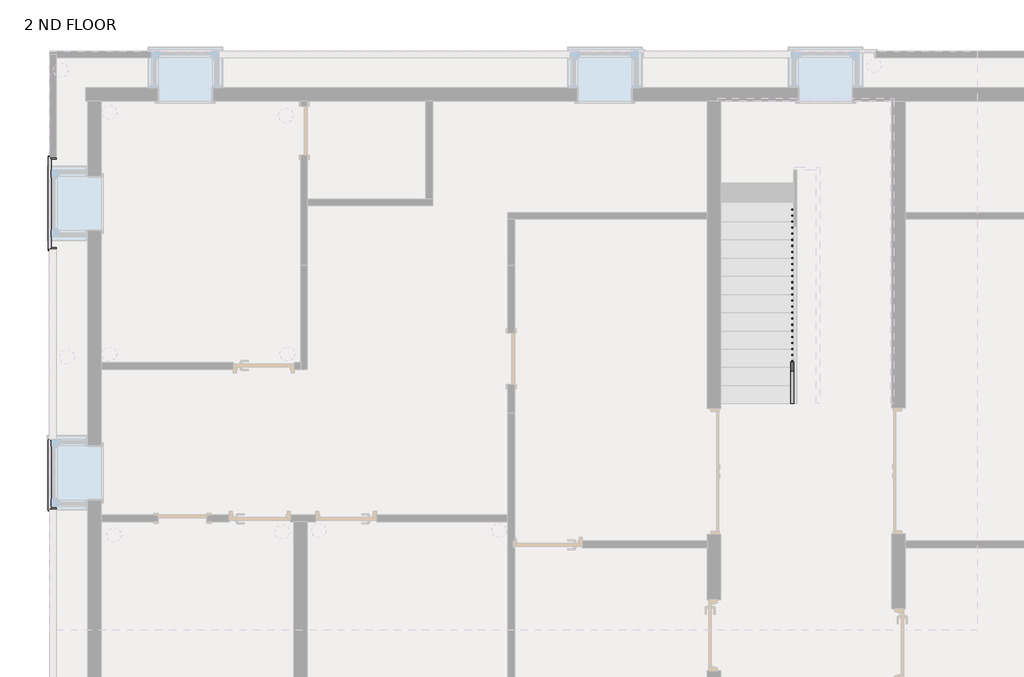
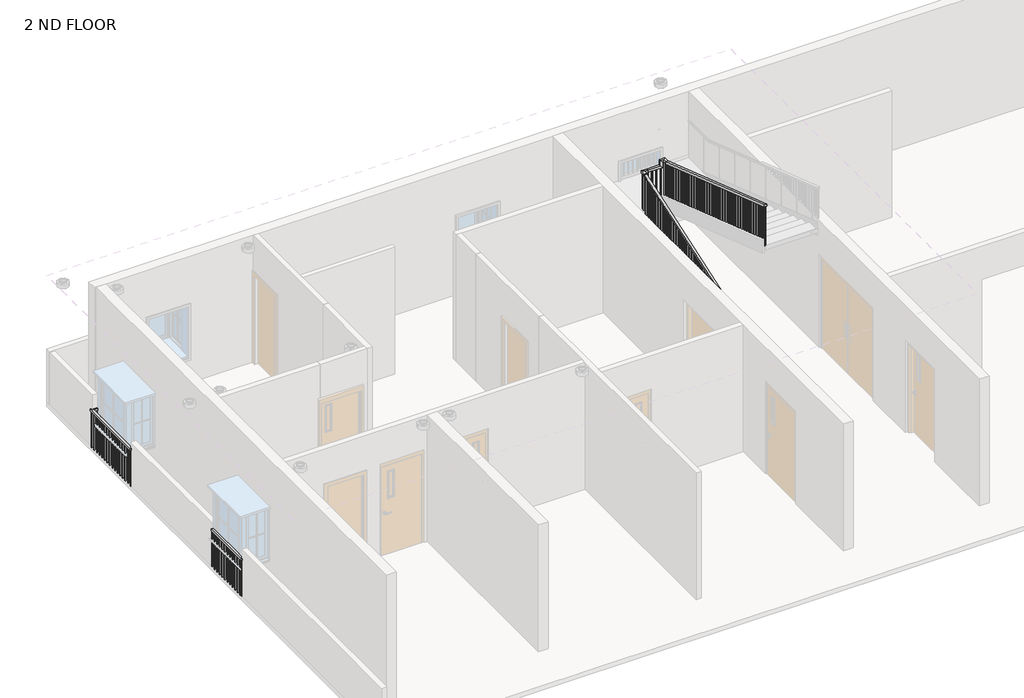
# One storey, part 4 of 7: 3 railings.
"""IFC4 building model written with IfcOpenShell, lengths in millimetres."""

from ifc_helpers import new_model, si_unit, frame, origin, place, context, project, spatial, polyline, outline, extrude, faceted_brep, element, save

model = new_model("IFC4")

# Units and contexts
model_context = context("Model", 3, world=origin())
ifc_project = project(units=[si_unit("LENGTHUNIT", "METRE", prefix="MILLI")], contexts=[model_context])

# Site, building, storey
site = spatial("IfcSite", under=ifc_project)
building = spatial("IfcBuilding", under=site)
storey = spatial("IfcBuildingStorey", under=building, Name="2 ND FLOOR", Elevation=6400.8)

# Railings
placement = place(None, origin())
element("IfcRailing", 1, ObjectType="Handrail - Rectangular", at=placement, inside=storey, context=model_context, shape_type="SolidModel", body=[
    faceted_brep([(-680.3987998, 2564.5067329, 7418.6142857), (-680.3987998, 2564.5067329, 7364.9699957), (-629.5987998, 2564.5067329, 7364.9699957), (-629.5987998, 2564.5067329, 7418.6142857), (-680.3987998, 6450.7067329, 8737.1464286), (-680.3987998, 6501.5067329, 8700.7378529), (-629.5987998, 6501.5067329, 8700.7378529), (-629.5987998, 6450.7067329, 8737.1464286), (-553.3987998, 6577.7067329, 8712.2), (-553.3987998, 6577.7067329, 8763.0), (-273.9987915, 6577.7067329, 8763.0), (-223.1987915, 6577.7067329, 8712.2), (-553.3987998, 6526.9067329, 8712.2), (-223.1987915, 6526.9067329, 8712.2), (-553.3987998, 6526.9067329, 8763.0), (-273.9987915, 6526.9067329, 8763.0), (-146.9987915, 2564.5067329, 10210.8), (-197.7987915, 2564.5067329, 10210.8), (-197.7987915, 2564.5067329, 10157.15571), (-146.9987915, 2564.5067329, 10157.15571), (-146.9987915, 6442.3235624, 8841.4678571), (-146.9987915, 6450.7067329, 8892.2678571), (-197.7987915, 6442.3235624, 8841.4678571), (-197.7987915, 6450.7067329, 8892.2678571), (-680.3987998, 6450.7067329, 8763.0), (-680.3987998, 6501.5067329, 8712.2), (-629.5987998, 6501.5067329, 8712.2), (-629.5987998, 6450.7067329, 8763.0), (-680.3987998, 6577.7067329, 8763.0), (-680.3987998, 6577.7067329, 8712.2), (-629.5987998, 6526.9067329, 8712.2), (-629.5987998, 6526.9067329, 8763.0), (-273.9987915, 6577.7067329, 8892.2678571), (-223.1987915, 6577.7067329, 8841.4678571), (-223.1987915, 6526.9067329, 8841.4678571), (-273.9987915, 6526.9067329, 8892.2678571), (-146.9987915, 6577.7067329, 8892.2678571), (-146.9987915, 6577.7067329, 8841.4678571), (-197.7987915, 6526.9067329, 8841.4678571), (-197.7987915, 6526.9067329, 8892.2678571)], [[[0, 1, 2, 3]], [[1, 0, 4, 5]], [[2, 1, 5, 6]], [[3, 2, 6, 7]], [[0, 3, 7, 4]], [[8, 9, 10, 11]], [[12, 8, 11, 13]], [[14, 12, 13, 15]], [[9, 14, 15, 10]], [[16, 17, 18, 19]], [[20, 21, 16, 19]], [[22, 20, 19, 18]], [[23, 22, 18, 17]], [[21, 23, 17, 16]], [[5, 4, 24, 25]], [[6, 5, 25, 26]], [[7, 6, 26, 27]], [[4, 7, 27, 24]], [[25, 24, 28, 29]], [[26, 25, 29, 30]], [[27, 26, 30, 31]], [[24, 27, 31, 28]], [[29, 28, 9, 8]], [[30, 29, 8, 12]], [[31, 30, 12, 14]], [[28, 31, 14, 9]], [[11, 10, 32, 33]], [[13, 11, 33, 34]], [[15, 13, 34, 35]], [[10, 15, 35, 32]], [[33, 32, 36, 37]], [[34, 33, 37, 38]], [[35, 34, 38, 39]], [[32, 35, 39, 36]], [[37, 36, 21, 20]], [[38, 37, 20, 22]], [[39, 38, 22, 23]], [[36, 39, 23, 21]]]),
    extrude(outline(polyline([(2580.3817329, 10151.7695493), (2599.4317329, 10145.3061565), (2599.4317329, 9192.9857143), (2580.3817329, 9192.9857143), (2580.3817329, 10151.7695493)])), frame((-181.9237915, 0.0, 0.0), z_axis=(1.0, 0.0, 0.0), x_axis=(0.0, 1.0, 0.0)), (0.0, 0.0, 1.0), 19.05),
    extrude(outline(polyline([(2681.9817329, 10117.2981207), (2701.0317329, 10110.8347279), (2701.0317329, 9192.9857143), (2681.9817329, 9192.9857143), (2681.9817329, 10117.2981207)])), frame((-181.9237915, 0.0, 0.0), z_axis=(1.0, 0.0, 0.0), x_axis=(0.0, 1.0, 0.0)), (0.0, 0.0, 1.0), 19.05),
    extrude(outline(polyline([(2783.5817329, 10082.8266922), (2802.6317329, 10076.3632993), (2802.6317329, 9192.9857143), (2783.5817329, 9192.9857143), (2783.5817329, 10082.8266922)])), frame((-181.9237915, 0.0, 0.0), z_axis=(1.0, 0.0, 0.0), x_axis=(0.0, 1.0, 0.0)), (0.0, 0.0, 1.0), 19.05),
    extrude(outline(polyline([(2885.1817329, 10048.3552636), (2904.2317329, 10041.8918707), (2904.2317329, 9089.5714286), (2885.1817329, 9089.5714286), (2885.1817329, 10048.3552636)])), frame((-181.9237915, 0.0, 0.0), z_axis=(1.0, 0.0, 0.0), x_axis=(0.0, 1.0, 0.0)), (0.0, 0.0, 1.0), 19.05),
    extrude(outline(polyline([(2986.7817329, 10013.883835), (3005.8317329, 10007.4204422), (3005.8317329, 9089.5714286), (2986.7817329, 9089.5714286), (2986.7817329, 10013.883835)])), frame((-181.9237915, 0.0, 0.0), z_axis=(1.0, 0.0, 0.0), x_axis=(0.0, 1.0, 0.0)), (0.0, 0.0, 1.0), 19.05),
    extrude(outline(polyline([(3088.3817329, 9979.4124065), (3107.4317329, 9972.9490136), (3107.4317329, 9089.5714286), (3088.3817329, 9089.5714286), (3088.3817329, 9979.4124065)])), frame((-181.9237915, 0.0, 0.0), z_axis=(1.0, 0.0, 0.0), x_axis=(0.0, 1.0, 0.0)), (0.0, 0.0, 1.0), 19.05),
    extrude(outline(polyline([(3189.9817329, 9944.9409779), (3209.0317329, 9938.477585), (3209.0317329, 8986.1571429), (3189.9817329, 8986.1571429), (3189.9817329, 9944.9409779)])), frame((-181.9237915, 0.0, 0.0), z_axis=(1.0, 0.0, 0.0), x_axis=(0.0, 1.0, 0.0)), (0.0, 0.0, 1.0), 19.05),
    extrude(outline(polyline([(3291.5817329, 9910.4695493), (3310.6317329, 9904.0061565), (3310.6317329, 8986.1571429), (3291.5817329, 8986.1571429), (3291.5817329, 9910.4695493)])), frame((-181.9237915, 0.0, 0.0), z_axis=(1.0, 0.0, 0.0), x_axis=(0.0, 1.0, 0.0)), (0.0, 0.0, 1.0), 19.05),
    extrude(outline(polyline([(3393.1817329, 9875.9981207), (3412.2317329, 9869.5347279), (3412.2317329, 8986.1571429), (3393.1817329, 8986.1571429), (3393.1817329, 9875.9981207)])), frame((-181.9237915, 0.0, 0.0), z_axis=(1.0, 0.0, 0.0), x_axis=(0.0, 1.0, 0.0)), (0.0, 0.0, 1.0), 19.05),
    extrude(outline(polyline([(3494.7817329, 9841.5266922), (3513.8317329, 9835.0632993), (3513.8317329, 8882.7428571), (3494.7817329, 8882.7428571), (3494.7817329, 9841.5266922)])), frame((-181.9237915, 0.0, 0.0), z_axis=(1.0, 0.0, 0.0), x_axis=(0.0, 1.0, 0.0)), (0.0, 0.0, 1.0), 19.05),
    extrude(outline(polyline([(3596.3817329, 9807.0552636), (3615.4317329, 9800.5918707), (3615.4317329, 8882.7428571), (3596.3817329, 8882.7428571), (3596.3817329, 9807.0552636)])), frame((-181.9237915, 0.0, 0.0), z_axis=(1.0, 0.0, 0.0), x_axis=(0.0, 1.0, 0.0)), (0.0, 0.0, 1.0), 19.05),
    extrude(outline(polyline([(3697.9817329, 9772.583835), (3717.0317329, 9766.1204422), (3717.0317329, 8882.7428571), (3697.9817329, 8882.7428571), (3697.9817329, 9772.583835)])), frame((-181.9237915, 0.0, 0.0), z_axis=(1.0, 0.0, 0.0), x_axis=(0.0, 1.0, 0.0)), (0.0, 0.0, 1.0), 19.05),
    extrude(outline(polyline([(3799.5817329, 9738.1124065), (3818.6317329, 9731.6490136), (3818.6317329, 8779.3285714), (3799.5817329, 8779.3285714), (3799.5817329, 9738.1124065)])), frame((-181.9237915, 0.0, 0.0), z_axis=(1.0, 0.0, 0.0), x_axis=(0.0, 1.0, 0.0)), (0.0, 0.0, 1.0), 19.05),
    extrude(outline(polyline([(3901.1817329, 9703.6409779), (3920.2317329, 9697.177585), (3920.2317329, 8779.3285714), (3901.1817329, 8779.3285714), (3901.1817329, 9703.6409779)])), frame((-181.9237915, 0.0, 0.0), z_axis=(1.0, 0.0, 0.0), x_axis=(0.0, 1.0, 0.0)), (0.0, 0.0, 1.0), 19.05),
    extrude(outline(polyline([(4002.7817329, 9669.1695493), (4021.8317329, 9662.7061565), (4021.8317329, 8779.3285714), (4002.7817329, 8779.3285714), (4002.7817329, 9669.1695493)])), frame((-181.9237915, 0.0, 0.0), z_axis=(1.0, 0.0, 0.0), x_axis=(0.0, 1.0, 0.0)), (0.0, 0.0, 1.0), 19.05),
    extrude(outline(polyline([(4104.3817329, 9634.6981207), (4123.4317329, 9628.2347279), (4123.4317329, 8675.9142857), (4104.3817329, 8675.9142857), (4104.3817329, 9634.6981207)])), frame((-181.9237915, 0.0, 0.0), z_axis=(1.0, 0.0, 0.0), x_axis=(0.0, 1.0, 0.0)), (0.0, 0.0, 1.0), 19.05),
    extrude(outline(polyline([(4205.9817329, 9600.2266922), (4225.0317329, 9593.7632993), (4225.0317329, 8675.9142857), (4205.9817329, 8675.9142857), (4205.9817329, 9600.2266922)])), frame((-181.9237915, 0.0, 0.0), z_axis=(1.0, 0.0, 0.0), x_axis=(0.0, 1.0, 0.0)), (0.0, 0.0, 1.0), 19.05),
    extrude(outline(polyline([(4307.5817329, 9565.7552636), (4326.6317329, 9559.2918707), (4326.6317329, 8675.9142857), (4307.5817329, 8675.9142857), (4307.5817329, 9565.7552636)])), frame((-181.9237915, 0.0, 0.0), z_axis=(1.0, 0.0, 0.0), x_axis=(0.0, 1.0, 0.0)), (0.0, 0.0, 1.0), 19.05),
    extrude(outline(polyline([(4409.1817329, 9531.283835), (4428.2317329, 9524.8204422), (4428.2317329, 8572.5), (4409.1817329, 8572.5), (4409.1817329, 9531.283835)])), frame((-181.9237915, 0.0, 0.0), z_axis=(1.0, 0.0, 0.0), x_axis=(0.0, 1.0, 0.0)), (0.0, 0.0, 1.0), 19.05),
    extrude(outline(polyline([(4510.7817329, 9496.8124065), (4529.8317329, 9490.3490136), (4529.8317329, 8572.5), (4510.7817329, 8572.5), (4510.7817329, 9496.8124065)])), frame((-181.9237915, 0.0, 0.0), z_axis=(1.0, 0.0, 0.0), x_axis=(0.0, 1.0, 0.0)), (0.0, 0.0, 1.0), 19.05),
    extrude(outline(polyline([(4612.3817329, 9462.3409779), (4631.4317329, 9455.877585), (4631.4317329, 8572.5), (4612.3817329, 8572.5), (4612.3817329, 9462.3409779)])), frame((-181.9237915, 0.0, 0.0), z_axis=(1.0, 0.0, 0.0), x_axis=(0.0, 1.0, 0.0)), (0.0, 0.0, 1.0), 19.05),
    extrude(outline(polyline([(4713.9817329, 9427.8695493), (4733.0317329, 9421.4061565), (4733.0317329, 8469.0857143), (4713.9817329, 8469.0857143), (4713.9817329, 9427.8695493)])), frame((-181.9237915, 0.0, 0.0), z_axis=(1.0, 0.0, 0.0), x_axis=(0.0, 1.0, 0.0)), (0.0, 0.0, 1.0), 19.05),
    extrude(outline(polyline([(4815.5817329, 9393.3981207), (4834.6317329, 9386.9347279), (4834.6317329, 8469.0857143), (4815.5817329, 8469.0857143), (4815.5817329, 9393.3981207)])), frame((-181.9237915, 0.0, 0.0), z_axis=(1.0, 0.0, 0.0), x_axis=(0.0, 1.0, 0.0)), (0.0, 0.0, 1.0), 19.05),
    extrude(outline(polyline([(4917.1817329, 9358.9266922), (4936.2317329, 9352.4632993), (4936.2317329, 8469.0857143), (4917.1817329, 8469.0857143), (4917.1817329, 9358.9266922)])), frame((-181.9237915, 0.0, 0.0), z_axis=(1.0, 0.0, 0.0), x_axis=(0.0, 1.0, 0.0)), (0.0, 0.0, 1.0), 19.05),
    extrude(outline(polyline([(5018.7817329, 9324.4552636), (5037.8317329, 9317.9918707), (5037.8317329, 8365.6714286), (5018.7817329, 8365.6714286), (5018.7817329, 9324.4552636)])), frame((-181.9237915, 0.0, 0.0), z_axis=(1.0, 0.0, 0.0), x_axis=(0.0, 1.0, 0.0)), (0.0, 0.0, 1.0), 19.05),
    extrude(outline(polyline([(5120.3817329, 9289.983835), (5139.4317329, 9283.5204422), (5139.4317329, 8365.6714286), (5120.3817329, 8365.6714286), (5120.3817329, 9289.983835)])), frame((-181.9237915, 0.0, 0.0), z_axis=(1.0, 0.0, 0.0), x_axis=(0.0, 1.0, 0.0)), (0.0, 0.0, 1.0), 19.05),
    extrude(outline(polyline([(5221.9817329, 9255.5124065), (5241.0317329, 9249.0490136), (5241.0317329, 8365.6714286), (5221.9817329, 8365.6714286), (5221.9817329, 9255.5124065)])), frame((-181.9237915, 0.0, 0.0), z_axis=(1.0, 0.0, 0.0), x_axis=(0.0, 1.0, 0.0)), (0.0, 0.0, 1.0), 19.05),
    extrude(outline(polyline([(5323.5817329, 9221.0409779), (5342.6317329, 9214.577585), (5342.6317329, 8262.2571429), (5323.5817329, 8262.2571429), (5323.5817329, 9221.0409779)])), frame((-181.9237915, 0.0, 0.0), z_axis=(1.0, 0.0, 0.0), x_axis=(0.0, 1.0, 0.0)), (0.0, 0.0, 1.0), 19.05),
    extrude(outline(polyline([(5425.1817329, 9186.5695493), (5444.2317329, 9180.1061565), (5444.2317329, 8262.2571429), (5425.1817329, 8262.2571429), (5425.1817329, 9186.5695493)])), frame((-181.9237915, 0.0, 0.0), z_axis=(1.0, 0.0, 0.0), x_axis=(0.0, 1.0, 0.0)), (0.0, 0.0, 1.0), 19.05),
    extrude(outline(polyline([(5526.7817329, 9152.0981207), (5545.8317329, 9145.6347279), (5545.8317329, 8262.2571429), (5526.7817329, 8262.2571429), (5526.7817329, 9152.0981207)])), frame((-181.9237915, 0.0, 0.0), z_axis=(1.0, 0.0, 0.0), x_axis=(0.0, 1.0, 0.0)), (0.0, 0.0, 1.0), 19.05),
    extrude(outline(polyline([(5628.3817329, 9117.6266922), (5647.4317329, 9111.1632993), (5647.4317329, 8158.8428571), (5628.3817329, 8158.8428571), (5628.3817329, 9117.6266922)])), frame((-181.9237915, 0.0, 0.0), z_axis=(1.0, 0.0, 0.0), x_axis=(0.0, 1.0, 0.0)), (0.0, 0.0, 1.0), 19.05),
    extrude(outline(polyline([(5729.9817329, 9083.1552636), (5749.0317329, 9076.6918707), (5749.0317329, 8158.8428571), (5729.9817329, 8158.8428571), (5729.9817329, 9083.1552636)])), frame((-181.9237915, 0.0, 0.0), z_axis=(1.0, 0.0, 0.0), x_axis=(0.0, 1.0, 0.0)), (0.0, 0.0, 1.0), 19.05),
    extrude(outline(polyline([(5831.5817329, 9048.683835), (5850.6317329, 9042.2204422), (5850.6317329, 8158.8428571), (5831.5817329, 8158.8428571), (5831.5817329, 9048.683835)])), frame((-181.9237915, 0.0, 0.0), z_axis=(1.0, 0.0, 0.0), x_axis=(0.0, 1.0, 0.0)), (0.0, 0.0, 1.0), 19.05),
    extrude(outline(polyline([(5933.1817329, 9014.2124065), (5952.2317329, 9007.7490136), (5952.2317329, 8055.4285714), (5933.1817329, 8055.4285714), (5933.1817329, 9014.2124065)])), frame((-181.9237915, 0.0, 0.0), z_axis=(1.0, 0.0, 0.0), x_axis=(0.0, 1.0, 0.0)), (0.0, 0.0, 1.0), 19.05),
    extrude(outline(polyline([(6034.7817329, 8979.7409779), (6053.8317329, 8973.277585), (6053.8317329, 8055.4285714), (6034.7817329, 8055.4285714), (6034.7817329, 8979.7409779)])), frame((-181.9237915, 0.0, 0.0), z_axis=(1.0, 0.0, 0.0), x_axis=(0.0, 1.0, 0.0)), (0.0, 0.0, 1.0), 19.05),
    extrude(outline(polyline([(6136.3817329, 8945.2695493), (6155.4317329, 8938.8061565), (6155.4317329, 8055.4285714), (6136.3817329, 8055.4285714), (6136.3817329, 8945.2695493)])), frame((-181.9237915, 0.0, 0.0), z_axis=(1.0, 0.0, 0.0), x_axis=(0.0, 1.0, 0.0)), (0.0, 0.0, 1.0), 19.05),
    extrude(outline(polyline([(6237.9817329, 8910.7981207), (6257.0317329, 8904.3347279), (6257.0317329, 7952.0142857), (6237.9817329, 7952.0142857), (6237.9817329, 8910.7981207)])), frame((-181.9237915, 0.0, 0.0), z_axis=(1.0, 0.0, 0.0), x_axis=(0.0, 1.0, 0.0)), (0.0, 0.0, 1.0), 19.05),
    extrude(outline(polyline([(6339.5817329, 8876.3266922), (6358.6317329, 8869.8632993), (6358.6317329, 7952.0142857), (6339.5817329, 7952.0142857), (6339.5817329, 8876.3266922)])), frame((-181.9237915, 0.0, 0.0), z_axis=(1.0, 0.0, 0.0), x_axis=(0.0, 1.0, 0.0)), (0.0, 0.0, 1.0), 19.05),
    extrude(outline(polyline([(6441.1817329, 8841.8552636), (6460.2317329, 8835.3918707), (6460.2317329, 7952.0142857), (6441.1817329, 7952.0142857), (6441.1817329, 8841.8552636)])), frame((-181.9237915, 0.0, 0.0), z_axis=(1.0, 0.0, 0.0), x_axis=(0.0, 1.0, 0.0)), (0.0, 0.0, 1.0), 19.05),
    extrude(outline(polyline([(-258.1237998, 6542.7817329), (-258.1237998, 6561.8317329), (-239.0737998, 6561.8317329), (-239.0737998, 6542.7817329), (-258.1237998, 6542.7817329)])), frame((0.0, 0.0, 7848.6), z_axis=(0.0, 0.0, 1.0), x_axis=(1.0, 0.0, 0.0)), (0.0, 0.0, 1.0), 992.8678571),
    extrude(outline(polyline([(-359.7237998, 6542.7817329), (-359.7237998, 6561.8317329), (-340.6737998, 6561.8317329), (-340.6737998, 6542.7817329), (-359.7237998, 6542.7817329)])), frame((0.0, 0.0, 7848.6), z_axis=(0.0, 0.0, 1.0), x_axis=(1.0, 0.0, 0.0)), (0.0, 0.0, 1.0), 863.6),
    extrude(outline(polyline([(-461.3237998, 6542.7817329), (-461.3237998, 6561.8317329), (-442.2737998, 6561.8317329), (-442.2737998, 6542.7817329), (-461.3237998, 6542.7817329)])), frame((0.0, 0.0, 7848.6), z_axis=(0.0, 0.0, 1.0), x_axis=(1.0, 0.0, 0.0)), (0.0, 0.0, 1.0), 863.6),
    extrude(outline(polyline([(-562.9237998, 6542.7817329), (-562.9237998, 6561.8317329), (-543.8737998, 6561.8317329), (-543.8737998, 6542.7817329), (-562.9237998, 6542.7817329)])), frame((0.0, 0.0, 7848.6), z_axis=(0.0, 0.0, 1.0), x_axis=(1.0, 0.0, 0.0)), (0.0, 0.0, 1.0), 863.6),
    extrude(outline(polyline([(-645.4737998, 6517.3817329), (-664.5237998, 6517.3817329), (-664.5237998, 6536.4317329), (-645.4737998, 6536.4317329), (-645.4737998, 6517.3817329)])), frame((0.0, 0.0, 7848.6), z_axis=(0.0, 0.0, 1.0), x_axis=(1.0, 0.0, 0.0)), (0.0, 0.0, 1.0), 863.6),
    extrude(outline(polyline([(6415.7817329, 8671.652585), (6434.8317329, 8678.1159779), (6434.8317329, 7745.1857143), (6415.7817329, 7745.1857143), (6415.7817329, 8671.652585)])), frame((-664.5237998, 0.0, 0.0), z_axis=(1.0, 0.0, 0.0), x_axis=(0.0, 1.0, 0.0)), (0.0, 0.0, 1.0), 19.05),
    extrude(outline(polyline([(6314.1817329, 8637.1811565), (6333.2317329, 8643.6445493), (6333.2317329, 7745.1857143), (6314.1817329, 7745.1857143), (6314.1817329, 8637.1811565)])), frame((-664.5237998, 0.0, 0.0), z_axis=(1.0, 0.0, 0.0), x_axis=(0.0, 1.0, 0.0)), (0.0, 0.0, 1.0), 19.05),
    extrude(outline(polyline([(6212.5817329, 8602.7097279), (6231.6317329, 8609.1731207), (6231.6317329, 7745.1857143), (6212.5817329, 7745.1857143), (6212.5817329, 8602.7097279)])), frame((-664.5237998, 0.0, 0.0), z_axis=(1.0, 0.0, 0.0), x_axis=(0.0, 1.0, 0.0)), (0.0, 0.0, 1.0), 19.05),
    extrude(outline(polyline([(6110.9817329, 8568.2382993), (6130.0317329, 8574.7016922), (6130.0317329, 7641.7714286), (6110.9817329, 7641.7714286), (6110.9817329, 8568.2382993)])), frame((-664.5237998, 0.0, 0.0), z_axis=(1.0, 0.0, 0.0), x_axis=(0.0, 1.0, 0.0)), (0.0, 0.0, 1.0), 19.05),
    extrude(outline(polyline([(6009.3817329, 8533.7668707), (6028.4317329, 8540.2302636), (6028.4317329, 7641.7714286), (6009.3817329, 7641.7714286), (6009.3817329, 8533.7668707)])), frame((-664.5237998, 0.0, 0.0), z_axis=(1.0, 0.0, 0.0), x_axis=(0.0, 1.0, 0.0)), (0.0, 0.0, 1.0), 19.05),
    extrude(outline(polyline([(5907.7817329, 8499.2954422), (5926.8317329, 8505.758835), (5926.8317329, 7641.7714286), (5907.7817329, 7641.7714286), (5907.7817329, 8499.2954422)])), frame((-664.5237998, 0.0, 0.0), z_axis=(1.0, 0.0, 0.0), x_axis=(0.0, 1.0, 0.0)), (0.0, 0.0, 1.0), 19.05),
    extrude(outline(polyline([(5806.1817329, 8464.8240136), (5825.2317329, 8471.2874065), (5825.2317329, 7538.3571429), (5806.1817329, 7538.3571429), (5806.1817329, 8464.8240136)])), frame((-664.5237998, 0.0, 0.0), z_axis=(1.0, 0.0, 0.0), x_axis=(0.0, 1.0, 0.0)), (0.0, 0.0, 1.0), 19.05),
    extrude(outline(polyline([(5704.5817329, 8430.352585), (5723.6317329, 8436.8159779), (5723.6317329, 7538.3571429), (5704.5817329, 7538.3571429), (5704.5817329, 8430.352585)])), frame((-664.5237998, 0.0, 0.0), z_axis=(1.0, 0.0, 0.0), x_axis=(0.0, 1.0, 0.0)), (0.0, 0.0, 1.0), 19.05),
    extrude(outline(polyline([(5602.9817329, 8395.8811565), (5622.0317329, 8402.3445493), (5622.0317329, 7538.3571429), (5602.9817329, 7538.3571429), (5602.9817329, 8395.8811565)])), frame((-664.5237998, 0.0, 0.0), z_axis=(1.0, 0.0, 0.0), x_axis=(0.0, 1.0, 0.0)), (0.0, 0.0, 1.0), 19.05),
    extrude(outline(polyline([(5501.3817329, 8361.4097279), (5520.4317329, 8367.8731207), (5520.4317329, 7434.9428571), (5501.3817329, 7434.9428571), (5501.3817329, 8361.4097279)])), frame((-664.5237998, 0.0, 0.0), z_axis=(1.0, 0.0, 0.0), x_axis=(0.0, 1.0, 0.0)), (0.0, 0.0, 1.0), 19.05),
    extrude(outline(polyline([(5399.7817329, 8326.9382993), (5418.8317329, 8333.4016922), (5418.8317329, 7434.9428571), (5399.7817329, 7434.9428571), (5399.7817329, 8326.9382993)])), frame((-664.5237998, 0.0, 0.0), z_axis=(1.0, 0.0, 0.0), x_axis=(0.0, 1.0, 0.0)), (0.0, 0.0, 1.0), 19.05),
    extrude(outline(polyline([(5298.1817329, 8292.4668707), (5317.2317329, 8298.9302636), (5317.2317329, 7434.9428571), (5298.1817329, 7434.9428571), (5298.1817329, 8292.4668707)])), frame((-664.5237998, 0.0, 0.0), z_axis=(1.0, 0.0, 0.0), x_axis=(0.0, 1.0, 0.0)), (0.0, 0.0, 1.0), 19.05),
    extrude(outline(polyline([(5196.5817329, 8257.9954422), (5215.6317329, 8264.458835), (5215.6317329, 7331.5285714), (5196.5817329, 7331.5285714), (5196.5817329, 8257.9954422)])), frame((-664.5237998, 0.0, 0.0), z_axis=(1.0, 0.0, 0.0), x_axis=(0.0, 1.0, 0.0)), (0.0, 0.0, 1.0), 19.05),
    extrude(outline(polyline([(5094.9817329, 8223.5240136), (5114.0317329, 8229.9874065), (5114.0317329, 7331.5285714), (5094.9817329, 7331.5285714), (5094.9817329, 8223.5240136)])), frame((-664.5237998, 0.0, 0.0), z_axis=(1.0, 0.0, 0.0), x_axis=(0.0, 1.0, 0.0)), (0.0, 0.0, 1.0), 19.05),
    extrude(outline(polyline([(4993.3817329, 8189.052585), (5012.4317329, 8195.5159779), (5012.4317329, 7331.5285714), (4993.3817329, 7331.5285714), (4993.3817329, 8189.052585)])), frame((-664.5237998, 0.0, 0.0), z_axis=(1.0, 0.0, 0.0), x_axis=(0.0, 1.0, 0.0)), (0.0, 0.0, 1.0), 19.05),
    extrude(outline(polyline([(4891.7817329, 8154.5811565), (4910.8317329, 8161.0445493), (4910.8317329, 7228.1142857), (4891.7817329, 7228.1142857), (4891.7817329, 8154.5811565)])), frame((-664.5237998, 0.0, 0.0), z_axis=(1.0, 0.0, 0.0), x_axis=(0.0, 1.0, 0.0)), (0.0, 0.0, 1.0), 19.05),
    extrude(outline(polyline([(4790.1817329, 8120.1097279), (4809.2317329, 8126.5731207), (4809.2317329, 7228.1142857), (4790.1817329, 7228.1142857), (4790.1817329, 8120.1097279)])), frame((-664.5237998, 0.0, 0.0), z_axis=(1.0, 0.0, 0.0), x_axis=(0.0, 1.0, 0.0)), (0.0, 0.0, 1.0), 19.05),
    extrude(outline(polyline([(4688.5817329, 8085.6382993), (4707.6317329, 8092.1016922), (4707.6317329, 7228.1142857), (4688.5817329, 7228.1142857), (4688.5817329, 8085.6382993)])), frame((-664.5237998, 0.0, 0.0), z_axis=(1.0, 0.0, 0.0), x_axis=(0.0, 1.0, 0.0)), (0.0, 0.0, 1.0), 19.05),
    extrude(outline(polyline([(4586.9817329, 8051.1668707), (4606.0317329, 8057.6302636), (4606.0317329, 7124.7), (4586.9817329, 7124.7), (4586.9817329, 8051.1668707)])), frame((-664.5237998, 0.0, 0.0), z_axis=(1.0, 0.0, 0.0), x_axis=(0.0, 1.0, 0.0)), (0.0, 0.0, 1.0), 19.05),
    extrude(outline(polyline([(4485.3817329, 8016.6954422), (4504.4317329, 8023.158835), (4504.4317329, 7124.7), (4485.3817329, 7124.7), (4485.3817329, 8016.6954422)])), frame((-664.5237998, 0.0, 0.0), z_axis=(1.0, 0.0, 0.0), x_axis=(0.0, 1.0, 0.0)), (0.0, 0.0, 1.0), 19.05),
    extrude(outline(polyline([(4383.7817329, 7982.2240136), (4402.8317329, 7988.6874065), (4402.8317329, 7124.7), (4383.7817329, 7124.7), (4383.7817329, 7982.2240136)])), frame((-664.5237998, 0.0, 0.0), z_axis=(1.0, 0.0, 0.0), x_axis=(0.0, 1.0, 0.0)), (0.0, 0.0, 1.0), 19.05),
    extrude(outline(polyline([(4282.1817329, 7947.752585), (4301.2317329, 7954.2159779), (4301.2317329, 7021.2857143), (4282.1817329, 7021.2857143), (4282.1817329, 7947.752585)])), frame((-664.5237998, 0.0, 0.0), z_axis=(1.0, 0.0, 0.0), x_axis=(0.0, 1.0, 0.0)), (0.0, 0.0, 1.0), 19.05),
    extrude(outline(polyline([(4180.5817329, 7913.2811565), (4199.6317329, 7919.7445493), (4199.6317329, 7021.2857143), (4180.5817329, 7021.2857143), (4180.5817329, 7913.2811565)])), frame((-664.5237998, 0.0, 0.0), z_axis=(1.0, 0.0, 0.0), x_axis=(0.0, 1.0, 0.0)), (0.0, 0.0, 1.0), 19.05),
    extrude(outline(polyline([(4078.9817329, 7878.8097279), (4098.0317329, 7885.2731207), (4098.0317329, 7021.2857143), (4078.9817329, 7021.2857143), (4078.9817329, 7878.8097279)])), frame((-664.5237998, 0.0, 0.0), z_axis=(1.0, 0.0, 0.0), x_axis=(0.0, 1.0, 0.0)), (0.0, 0.0, 1.0), 19.05),
    extrude(outline(polyline([(3977.3817329, 7844.3382993), (3996.4317329, 7850.8016922), (3996.4317329, 6917.8714286), (3977.3817329, 6917.8714286), (3977.3817329, 7844.3382993)])), frame((-664.5237998, 0.0, 0.0), z_axis=(1.0, 0.0, 0.0), x_axis=(0.0, 1.0, 0.0)), (0.0, 0.0, 1.0), 19.05),
    extrude(outline(polyline([(3875.7817329, 7809.8668707), (3894.8317329, 7816.3302636), (3894.8317329, 6917.8714286), (3875.7817329, 6917.8714286), (3875.7817329, 7809.8668707)])), frame((-664.5237998, 0.0, 0.0), z_axis=(1.0, 0.0, 0.0), x_axis=(0.0, 1.0, 0.0)), (0.0, 0.0, 1.0), 19.05),
    extrude(outline(polyline([(3774.1817329, 7775.3954422), (3793.2317329, 7781.858835), (3793.2317329, 6917.8714286), (3774.1817329, 6917.8714286), (3774.1817329, 7775.3954422)])), frame((-664.5237998, 0.0, 0.0), z_axis=(1.0, 0.0, 0.0), x_axis=(0.0, 1.0, 0.0)), (0.0, 0.0, 1.0), 19.05),
    extrude(outline(polyline([(3672.5817329, 7740.9240136), (3691.6317329, 7747.3874065), (3691.6317329, 6814.4571429), (3672.5817329, 6814.4571429), (3672.5817329, 7740.9240136)])), frame((-664.5237998, 0.0, 0.0), z_axis=(1.0, 0.0, 0.0), x_axis=(0.0, 1.0, 0.0)), (0.0, 0.0, 1.0), 19.05),
    extrude(outline(polyline([(3570.9817329, 7706.452585), (3590.0317329, 7712.9159779), (3590.0317329, 6814.4571429), (3570.9817329, 6814.4571429), (3570.9817329, 7706.452585)])), frame((-664.5237998, 0.0, 0.0), z_axis=(1.0, 0.0, 0.0), x_axis=(0.0, 1.0, 0.0)), (0.0, 0.0, 1.0), 19.05),
    extrude(outline(polyline([(3469.3817329, 7671.9811565), (3488.4317329, 7678.4445493), (3488.4317329, 6814.4571429), (3469.3817329, 6814.4571429), (3469.3817329, 7671.9811565)])), frame((-664.5237998, 0.0, 0.0), z_axis=(1.0, 0.0, 0.0), x_axis=(0.0, 1.0, 0.0)), (0.0, 0.0, 1.0), 19.05),
    extrude(outline(polyline([(3367.7817329, 7637.5097279), (3386.8317329, 7643.9731207), (3386.8317329, 6711.0428571), (3367.7817329, 6711.0428571), (3367.7817329, 7637.5097279)])), frame((-664.5237998, 0.0, 0.0), z_axis=(1.0, 0.0, 0.0), x_axis=(0.0, 1.0, 0.0)), (0.0, 0.0, 1.0), 19.05),
    extrude(outline(polyline([(3266.1817329, 7603.0382993), (3285.2317329, 7609.5016922), (3285.2317329, 6711.0428571), (3266.1817329, 6711.0428571), (3266.1817329, 7603.0382993)])), frame((-664.5237998, 0.0, 0.0), z_axis=(1.0, 0.0, 0.0), x_axis=(0.0, 1.0, 0.0)), (0.0, 0.0, 1.0), 19.05),
    extrude(outline(polyline([(3164.5817329, 7568.5668707), (3183.6317329, 7575.0302636), (3183.6317329, 6711.0428571), (3164.5817329, 6711.0428571), (3164.5817329, 7568.5668707)])), frame((-664.5237998, 0.0, 0.0), z_axis=(1.0, 0.0, 0.0), x_axis=(0.0, 1.0, 0.0)), (0.0, 0.0, 1.0), 19.05),
    extrude(outline(polyline([(3062.9817329, 7534.0954422), (3082.0317329, 7540.558835), (3082.0317329, 6607.6285714), (3062.9817329, 6607.6285714), (3062.9817329, 7534.0954422)])), frame((-664.5237998, 0.0, 0.0), z_axis=(1.0, 0.0, 0.0), x_axis=(0.0, 1.0, 0.0)), (0.0, 0.0, 1.0), 19.05),
    extrude(outline(polyline([(2961.3817329, 7499.6240136), (2980.4317329, 7506.0874065), (2980.4317329, 6607.6285714), (2961.3817329, 6607.6285714), (2961.3817329, 7499.6240136)])), frame((-664.5237998, 0.0, 0.0), z_axis=(1.0, 0.0, 0.0), x_axis=(0.0, 1.0, 0.0)), (0.0, 0.0, 1.0), 19.05),
    extrude(outline(polyline([(2859.7817329, 7465.152585), (2878.8317329, 7471.6159779), (2878.8317329, 6607.6285714), (2859.7817329, 6607.6285714), (2859.7817329, 7465.152585)])), frame((-664.5237998, 0.0, 0.0), z_axis=(1.0, 0.0, 0.0), x_axis=(0.0, 1.0, 0.0)), (0.0, 0.0, 1.0), 19.05),
    extrude(outline(polyline([(2758.1817329, 7430.6811565), (2777.2317329, 7437.1445493), (2777.2317329, 6504.2142857), (2758.1817329, 6504.2142857), (2758.1817329, 7430.6811565)])), frame((-664.5237998, 0.0, 0.0), z_axis=(1.0, 0.0, 0.0), x_axis=(0.0, 1.0, 0.0)), (0.0, 0.0, 1.0), 19.05),
    extrude(outline(polyline([(2656.5817329, 7396.2097279), (2675.6317329, 7402.6731207), (2675.6317329, 6504.2142857), (2656.5817329, 6504.2142857), (2656.5817329, 7396.2097279)])), frame((-664.5237998, 0.0, 0.0), z_axis=(1.0, 0.0, 0.0), x_axis=(0.0, 1.0, 0.0)), (0.0, 0.0, 1.0), 19.05),
    extrude(outline(polyline([(-181.9237915, 6542.7817329), (-181.9237915, 6561.8317329), (-162.8737915, 6561.8317329), (-162.8737915, 6542.7817329), (-181.9237915, 6542.7817329)])), frame((0.0, 0.0, 7848.6), z_axis=(0.0, 0.0, 1.0), x_axis=(1.0, 0.0, 0.0)), (0.0, 0.0, 1.0), 992.8678571),
    extrude(outline(polyline([(-645.4737998, 6542.7817329), (-664.5237998, 6542.7817329), (-664.5237998, 6561.8317329), (-645.4737998, 6561.8317329), (-645.4737998, 6542.7817329)])), frame((0.0, 0.0, 7848.6), z_axis=(0.0, 0.0, 1.0), x_axis=(1.0, 0.0, 0.0)), (0.0, 0.0, 1.0), 863.6),
    extrude(outline(polyline([(2564.5067329, 10157.15571), (2583.5567329, 10150.6923172), (2583.5567329, 9192.9857143), (2564.5067329, 9192.9857143), (2564.5067329, 10157.15571)])), frame((-181.9237915, 0.0, 0.0), z_axis=(1.0, 0.0, 0.0), x_axis=(0.0, 1.0, 0.0)), (0.0, 0.0, 1.0), 19.05),
    extrude(outline(polyline([(2564.5067329, 7364.9699957), (2583.5567329, 7371.4333886), (2583.5567329, 6504.2142857), (2564.5067329, 6504.2142857), (2564.5067329, 7364.9699957)])), frame((-664.5237998, 0.0, 0.0), z_axis=(1.0, 0.0, 0.0), x_axis=(0.0, 1.0, 0.0)), (0.0, 0.0, 1.0), 19.05),
])
element("IfcRailing", 2, ObjectType="Handrail - Rectangular", at=placement, inside=storey, context=model_context, shape_type="SolidModel", body=[
    faceted_brep([(-13063.4067989, 1953.9604213, 7315.2), (-13063.4067989, 1953.9604213, 7264.4), (-13114.2067989, 1953.9604213, 7264.4), (-13114.2067989, 1953.9604213, 7315.2), (-13063.4067989, 818.2567339, 7315.2), (-13063.4067989, 818.2567339, 7264.4), (-13114.2067989, 767.4567339, 7264.4), (-13114.2067989, 767.4567339, 7315.2), (-12974.5067989, 818.2567339, 7315.2), (-12974.5067989, 767.4567339, 7315.2), (-12974.5067989, 767.4567339, 7264.4), (-12974.5067989, 818.2567339, 7264.4)], [[[0, 1, 2, 3]], [[1, 0, 4, 5]], [[2, 1, 5, 6]], [[3, 2, 6, 7]], [[0, 3, 7, 4]], [[8, 9, 10, 11]], [[5, 4, 8, 11]], [[6, 5, 11, 10]], [[7, 6, 10, 9]], [[4, 7, 9, 8]]]),
    extrude(outline(polyline([(-12996.7317989, 783.3317339), (-12996.7317989, 802.3817339), (-12977.6817989, 802.3817339), (-12977.6817989, 783.3317339), (-12996.7317989, 783.3317339)])), frame((0.0, 0.0, 6400.8), z_axis=(0.0, 0.0, 1.0), x_axis=(1.0, 0.0, 0.0)), (0.0, 0.0, 1.0), 863.6),
    extrude(outline(polyline([(-13098.3317989, 845.8854213), (-13079.2817989, 845.8854213), (-13079.2817989, 826.8354213), (-13098.3317989, 826.8354213), (-13098.3317989, 845.8854213)])), frame((0.0, 0.0, 6400.8), z_axis=(0.0, 0.0, 1.0), x_axis=(1.0, 0.0, 0.0)), (0.0, 0.0, 1.0), 863.6),
    extrude(outline(polyline([(-13098.3317989, 947.4854213), (-13079.2817989, 947.4854213), (-13079.2817989, 928.4354213), (-13098.3317989, 928.4354213), (-13098.3317989, 947.4854213)])), frame((0.0, 0.0, 6400.8), z_axis=(0.0, 0.0, 1.0), x_axis=(1.0, 0.0, 0.0)), (0.0, 0.0, 1.0), 863.6),
    extrude(outline(polyline([(-13098.3317989, 1049.0854213), (-13079.2817989, 1049.0854213), (-13079.2817989, 1030.0354213), (-13098.3317989, 1030.0354213), (-13098.3317989, 1049.0854213)])), frame((0.0, 0.0, 6400.8), z_axis=(0.0, 0.0, 1.0), x_axis=(1.0, 0.0, 0.0)), (0.0, 0.0, 1.0), 863.6),
    extrude(outline(polyline([(-13098.3317989, 1150.6854213), (-13079.2817989, 1150.6854213), (-13079.2817989, 1131.6354213), (-13098.3317989, 1131.6354213), (-13098.3317989, 1150.6854213)])), frame((0.0, 0.0, 6400.8), z_axis=(0.0, 0.0, 1.0), x_axis=(1.0, 0.0, 0.0)), (0.0, 0.0, 1.0), 863.6),
    extrude(outline(polyline([(-13098.3317989, 1252.2854213), (-13079.2817989, 1252.2854213), (-13079.2817989, 1233.2354213), (-13098.3317989, 1233.2354213), (-13098.3317989, 1252.2854213)])), frame((0.0, 0.0, 6400.8), z_axis=(0.0, 0.0, 1.0), x_axis=(1.0, 0.0, 0.0)), (0.0, 0.0, 1.0), 863.6),
    extrude(outline(polyline([(-13098.3317989, 1353.8854213), (-13079.2817989, 1353.8854213), (-13079.2817989, 1334.8354213), (-13098.3317989, 1334.8354213), (-13098.3317989, 1353.8854213)])), frame((0.0, 0.0, 6400.8), z_axis=(0.0, 0.0, 1.0), x_axis=(1.0, 0.0, 0.0)), (0.0, 0.0, 1.0), 863.6),
    extrude(outline(polyline([(-13098.3317989, 1455.4854213), (-13079.2817989, 1455.4854213), (-13079.2817989, 1436.4354213), (-13098.3317989, 1436.4354213), (-13098.3317989, 1455.4854213)])), frame((0.0, 0.0, 6400.8), z_axis=(0.0, 0.0, 1.0), x_axis=(1.0, 0.0, 0.0)), (0.0, 0.0, 1.0), 863.6),
    extrude(outline(polyline([(-13098.3317989, 1557.0854213), (-13079.2817989, 1557.0854213), (-13079.2817989, 1538.0354213), (-13098.3317989, 1538.0354213), (-13098.3317989, 1557.0854213)])), frame((0.0, 0.0, 6400.8), z_axis=(0.0, 0.0, 1.0), x_axis=(1.0, 0.0, 0.0)), (0.0, 0.0, 1.0), 863.6),
    extrude(outline(polyline([(-13098.3317989, 1658.6854213), (-13079.2817989, 1658.6854213), (-13079.2817989, 1639.6354213), (-13098.3317989, 1639.6354213), (-13098.3317989, 1658.6854213)])), frame((0.0, 0.0, 6400.8), z_axis=(0.0, 0.0, 1.0), x_axis=(1.0, 0.0, 0.0)), (0.0, 0.0, 1.0), 863.6),
    extrude(outline(polyline([(-13098.3317989, 1760.2854213), (-13079.2817989, 1760.2854213), (-13079.2817989, 1741.2354213), (-13098.3317989, 1741.2354213), (-13098.3317989, 1760.2854213)])), frame((0.0, 0.0, 6400.8), z_axis=(0.0, 0.0, 1.0), x_axis=(1.0, 0.0, 0.0)), (0.0, 0.0, 1.0), 863.6),
    extrude(outline(polyline([(-13098.3317989, 1861.8854213), (-13079.2817989, 1861.8854213), (-13079.2817989, 1842.8354213), (-13098.3317989, 1842.8354213), (-13098.3317989, 1861.8854213)])), frame((0.0, 0.0, 6400.8), z_axis=(0.0, 0.0, 1.0), x_axis=(1.0, 0.0, 0.0)), (0.0, 0.0, 1.0), 863.6),
    extrude(outline(polyline([(-13098.3317989, 802.3817339), (-13079.2817989, 802.3817339), (-13079.2817989, 783.3317339), (-13098.3317989, 783.3317339), (-13098.3317989, 802.3817339)])), frame((0.0, 0.0, 6400.8), z_axis=(0.0, 0.0, 1.0), x_axis=(1.0, 0.0, 0.0)), (0.0, 0.0, 1.0), 863.6),
    extrude(outline(polyline([(-13079.2817989, 1963.4854213), (-13079.2817989, 1944.4354213), (-13098.3317989, 1944.4354213), (-13098.3317989, 1963.4854213), (-13079.2817989, 1963.4854213)])), frame((0.0, 0.0, 6400.8), z_axis=(0.0, 0.0, 1.0), x_axis=(1.0, 0.0, 0.0)), (0.0, 0.0, 1.0), 863.6),
    extrude(outline(polyline([(-12993.5567989, 783.3317339), (-12993.5567989, 802.3817339), (-12974.5067989, 802.3817339), (-12974.5067989, 783.3317339), (-12993.5567989, 783.3317339)])), frame((0.0, 0.0, 6400.8), z_axis=(0.0, 0.0, 1.0), x_axis=(1.0, 0.0, 0.0)), (0.0, 0.0, 1.0), 863.6),
    extrude(outline(polyline([(-13062.8987925, 1963.4854213), (-13062.8987925, 1944.4354213), (-13081.9487925, 1944.4354213), (-13081.9487925, 1963.4854213), (-13062.8987925, 1963.4854213)])), frame((0.0, 0.0, 6400.8), z_axis=(0.0, 0.0, 1.0), x_axis=(1.0, 0.0, 0.0)), (0.0, 0.0, 1.0), 863.6),
])
element("IfcRailing", 3, ObjectType="Handrail - Rectangular", at=placement, inside=storey, context=model_context, shape_type="SolidModel", body=[
    faceted_brep([(-12973.9987925, 6656.8711337, 7315.2), (-12973.9987925, 6656.8711337, 7264.4), (-12973.9987925, 6707.6711337, 7264.4), (-12973.9987925, 6707.6711337, 7315.2), (-13062.8987925, 6656.8711337, 7315.2), (-13062.8987925, 6656.8711337, 7264.4), (-13113.6987925, 6707.6711337, 7264.4), (-13113.6987925, 6707.6711337, 7315.2), (-13062.8987925, 5180.1736362, 7315.2), (-13062.8987925, 5180.1736362, 7264.4), (-13113.6987925, 5129.3736362, 7264.4), (-13113.6987925, 5129.3736362, 7315.2), (-12973.9987925, 5180.1736362, 7315.2), (-12973.9987925, 5129.3736362, 7315.2), (-12973.9987925, 5129.3736362, 7264.4), (-12973.9987925, 5180.1736362, 7264.4)], [[[0, 1, 2, 3]], [[1, 0, 4, 5]], [[2, 1, 5, 6]], [[3, 2, 6, 7]], [[0, 3, 7, 4]], [[5, 4, 8, 9]], [[6, 5, 9, 10]], [[7, 6, 10, 11]], [[4, 7, 11, 8]], [[12, 13, 14, 15]], [[9, 8, 12, 15]], [[10, 9, 15, 14]], [[11, 10, 14, 13]], [[8, 11, 13, 12]]]),
    extrude(outline(polyline([(-12996.2237925, 5145.2486362), (-12996.2237925, 5164.2986362), (-12977.1737925, 5164.2986362), (-12977.1737925, 5145.2486362), (-12996.2237925, 5145.2486362)])), frame((0.0, 0.0, 6400.8), z_axis=(0.0, 0.0, 1.0), x_axis=(1.0, 0.0, 0.0)), (0.0, 0.0, 1.0), 863.6),
    extrude(outline(polyline([(-13097.8237925, 5167.7961337), (-13078.7737925, 5167.7961337), (-13078.7737925, 5148.7461337), (-13097.8237925, 5148.7461337), (-13097.8237925, 5167.7961337)])), frame((0.0, 0.0, 6400.8), z_axis=(0.0, 0.0, 1.0), x_axis=(1.0, 0.0, 0.0)), (0.0, 0.0, 1.0), 863.6),
    extrude(outline(polyline([(-13097.8237925, 5269.3961337), (-13078.7737925, 5269.3961337), (-13078.7737925, 5250.3461337), (-13097.8237925, 5250.3461337), (-13097.8237925, 5269.3961337)])), frame((0.0, 0.0, 6400.8), z_axis=(0.0, 0.0, 1.0), x_axis=(1.0, 0.0, 0.0)), (0.0, 0.0, 1.0), 863.6),
    extrude(outline(polyline([(-13097.8237925, 5370.9961337), (-13078.7737925, 5370.9961337), (-13078.7737925, 5351.9461337), (-13097.8237925, 5351.9461337), (-13097.8237925, 5370.9961337)])), frame((0.0, 0.0, 6400.8), z_axis=(0.0, 0.0, 1.0), x_axis=(1.0, 0.0, 0.0)), (0.0, 0.0, 1.0), 863.6),
    extrude(outline(polyline([(-13097.8237925, 5472.5961337), (-13078.7737925, 5472.5961337), (-13078.7737925, 5453.5461337), (-13097.8237925, 5453.5461337), (-13097.8237925, 5472.5961337)])), frame((0.0, 0.0, 6400.8), z_axis=(0.0, 0.0, 1.0), x_axis=(1.0, 0.0, 0.0)), (0.0, 0.0, 1.0), 863.6),
    extrude(outline(polyline([(-13097.8237925, 5574.1961337), (-13078.7737925, 5574.1961337), (-13078.7737925, 5555.1461337), (-13097.8237925, 5555.1461337), (-13097.8237925, 5574.1961337)])), frame((0.0, 0.0, 6400.8), z_axis=(0.0, 0.0, 1.0), x_axis=(1.0, 0.0, 0.0)), (0.0, 0.0, 1.0), 863.6),
    extrude(outline(polyline([(-13097.8237925, 5675.7961337), (-13078.7737925, 5675.7961337), (-13078.7737925, 5656.7461337), (-13097.8237925, 5656.7461337), (-13097.8237925, 5675.7961337)])), frame((0.0, 0.0, 6400.8), z_axis=(0.0, 0.0, 1.0), x_axis=(1.0, 0.0, 0.0)), (0.0, 0.0, 1.0), 863.6),
    extrude(outline(polyline([(-13097.8237925, 5777.3961337), (-13078.7737925, 5777.3961337), (-13078.7737925, 5758.3461337), (-13097.8237925, 5758.3461337), (-13097.8237925, 5777.3961337)])), frame((0.0, 0.0, 6400.8), z_axis=(0.0, 0.0, 1.0), x_axis=(1.0, 0.0, 0.0)), (0.0, 0.0, 1.0), 863.6),
    extrude(outline(polyline([(-13097.8237925, 5878.9961337), (-13078.7737925, 5878.9961337), (-13078.7737925, 5859.9461337), (-13097.8237925, 5859.9461337), (-13097.8237925, 5878.9961337)])), frame((0.0, 0.0, 6400.8), z_axis=(0.0, 0.0, 1.0), x_axis=(1.0, 0.0, 0.0)), (0.0, 0.0, 1.0), 863.6),
    extrude(outline(polyline([(-13097.8237925, 5980.5961337), (-13078.7737925, 5980.5961337), (-13078.7737925, 5961.5461337), (-13097.8237925, 5961.5461337), (-13097.8237925, 5980.5961337)])), frame((0.0, 0.0, 6400.8), z_axis=(0.0, 0.0, 1.0), x_axis=(1.0, 0.0, 0.0)), (0.0, 0.0, 1.0), 863.6),
    extrude(outline(polyline([(-13097.8237925, 6082.1961337), (-13078.7737925, 6082.1961337), (-13078.7737925, 6063.1461337), (-13097.8237925, 6063.1461337), (-13097.8237925, 6082.1961337)])), frame((0.0, 0.0, 6400.8), z_axis=(0.0, 0.0, 1.0), x_axis=(1.0, 0.0, 0.0)), (0.0, 0.0, 1.0), 863.6),
    extrude(outline(polyline([(-13097.8237925, 6183.7961337), (-13078.7737925, 6183.7961337), (-13078.7737925, 6164.7461337), (-13097.8237925, 6164.7461337), (-13097.8237925, 6183.7961337)])), frame((0.0, 0.0, 6400.8), z_axis=(0.0, 0.0, 1.0), x_axis=(1.0, 0.0, 0.0)), (0.0, 0.0, 1.0), 863.6),
    extrude(outline(polyline([(-13097.8237925, 6285.3961337), (-13078.7737925, 6285.3961337), (-13078.7737925, 6266.3461337), (-13097.8237925, 6266.3461337), (-13097.8237925, 6285.3961337)])), frame((0.0, 0.0, 6400.8), z_axis=(0.0, 0.0, 1.0), x_axis=(1.0, 0.0, 0.0)), (0.0, 0.0, 1.0), 863.6),
    extrude(outline(polyline([(-13097.8237925, 6386.9961337), (-13078.7737925, 6386.9961337), (-13078.7737925, 6367.9461337), (-13097.8237925, 6367.9461337), (-13097.8237925, 6386.9961337)])), frame((0.0, 0.0, 6400.8), z_axis=(0.0, 0.0, 1.0), x_axis=(1.0, 0.0, 0.0)), (0.0, 0.0, 1.0), 863.6),
    extrude(outline(polyline([(-13097.8237925, 6488.5961337), (-13078.7737925, 6488.5961337), (-13078.7737925, 6469.5461337), (-13097.8237925, 6469.5461337), (-13097.8237925, 6488.5961337)])), frame((0.0, 0.0, 6400.8), z_axis=(0.0, 0.0, 1.0), x_axis=(1.0, 0.0, 0.0)), (0.0, 0.0, 1.0), 863.6),
    extrude(outline(polyline([(-13097.8237925, 6590.1961337), (-13078.7737925, 6590.1961337), (-13078.7737925, 6571.1461337), (-13097.8237925, 6571.1461337), (-13097.8237925, 6590.1961337)])), frame((0.0, 0.0, 6400.8), z_axis=(0.0, 0.0, 1.0), x_axis=(1.0, 0.0, 0.0)), (0.0, 0.0, 1.0), 863.6),
    extrude(outline(polyline([(-13066.0737925, 6691.7961337), (-13066.0737925, 6672.7461337), (-13085.1237925, 6672.7461337), (-13085.1237925, 6691.7961337), (-13066.0737925, 6691.7961337)])), frame((0.0, 0.0, 6400.8), z_axis=(0.0, 0.0, 1.0), x_axis=(1.0, 0.0, 0.0)), (0.0, 0.0, 1.0), 863.6),
    extrude(outline(polyline([(-13097.8237925, 5164.2986362), (-13078.7737925, 5164.2986362), (-13078.7737925, 5145.2486362), (-13097.8237925, 5145.2486362), (-13097.8237925, 5164.2986362)])), frame((0.0, 0.0, 6400.8), z_axis=(0.0, 0.0, 1.0), x_axis=(1.0, 0.0, 0.0)), (0.0, 0.0, 1.0), 863.6),
    extrude(outline(polyline([(-13078.7737925, 6691.7961337), (-13078.7737925, 6672.7461337), (-13097.8237925, 6672.7461337), (-13097.8237925, 6691.7961337), (-13078.7737925, 6691.7961337)])), frame((0.0, 0.0, 6400.8), z_axis=(0.0, 0.0, 1.0), x_axis=(1.0, 0.0, 0.0)), (0.0, 0.0, 1.0), 863.6),
    extrude(outline(polyline([(-12993.0487925, 5145.2486362), (-12993.0487925, 5164.2986362), (-12973.9987925, 5164.2986362), (-12973.9987925, 5145.2486362), (-12993.0487925, 5145.2486362)])), frame((0.0, 0.0, 6400.8), z_axis=(0.0, 0.0, 1.0), x_axis=(1.0, 0.0, 0.0)), (0.0, 0.0, 1.0), 863.6),
    extrude(outline(polyline([(-12973.9987925, 6691.7961337), (-12973.9987925, 6672.7461337), (-12993.0487925, 6672.7461337), (-12993.0487925, 6691.7961337), (-12973.9987925, 6691.7961337)])), frame((0.0, 0.0, 6400.8), z_axis=(0.0, 0.0, 1.0), x_axis=(1.0, 0.0, 0.0)), (0.0, 0.0, 1.0), 863.6),
])

save(model, "model.ifc")

# Revit data of these elements
# Type "Handrail - Rectangular"
#   Assembly Code = "C2010400"
#   built-in parameter 1008612 = 0.0416667 (stored number, unit not read)
#   built-in parameter 1008611 = 0.0416667 (stored number, unit not read)
#   built-in parameter 1008609 = 0.333333 (stored number, unit not read)
#   built-in parameter 1008604 = 0.166667 (stored number, unit not read)
#   built-in parameter 1008603 = 0.166667 (stored number, unit not read)
#   Railing Height = 3' - 0"
#   built-in parameter 1008630 = 2
#   built-in parameter 1008610 = 2
#   built-in parameter 1008618 = Baluster - Square : 3/4"
# Elements 1, 2, 3 (IfcRailing, "Handrail - Rectangular")
#   Phase Created = New Construction
